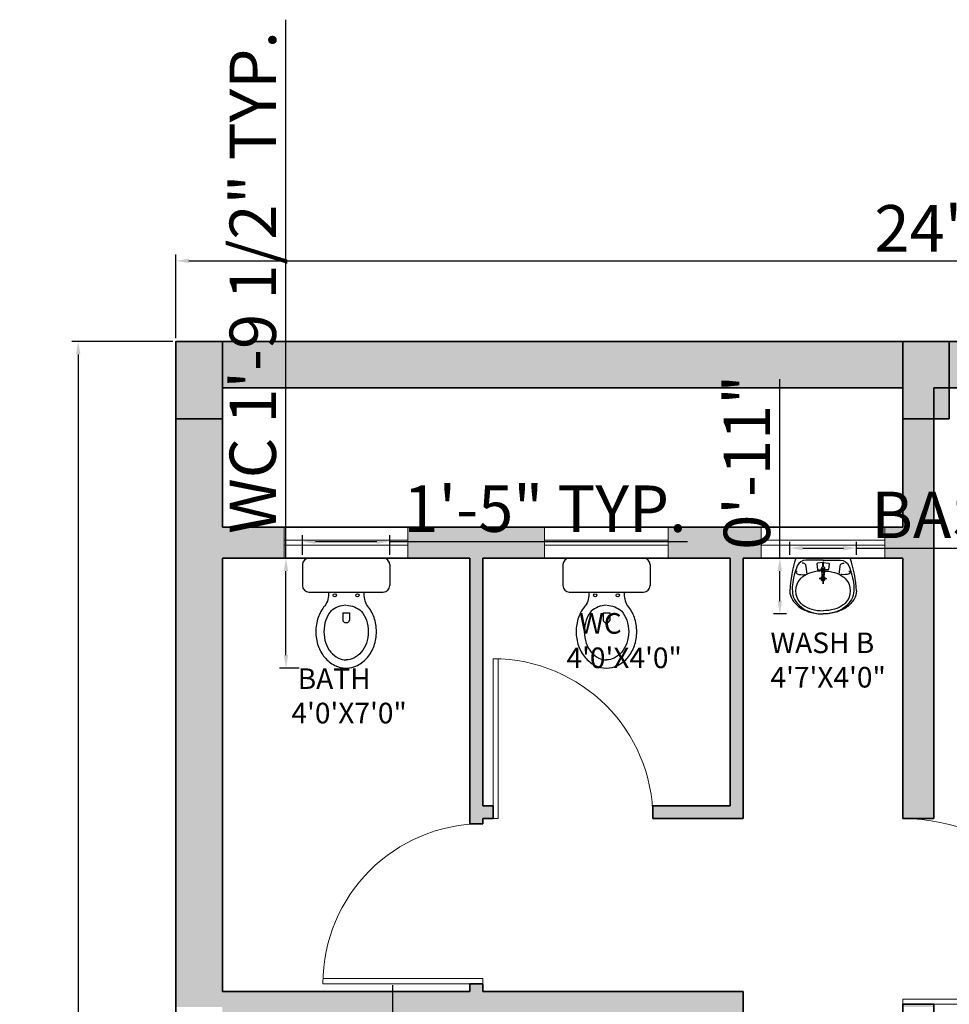
# Model space of a CAD drawing. Units: inches. Extents: x 3148 to 3962, y 1142 to 1671.
# Tile 3 of 9: x 3164 to 3344, y 1426 to 1617. Entities that reach past the tile are written whole.
import ezdxf

# ---------------------------------------------------------------- set-up
doc = ezdxf.new("R2010")
doc.units = ezdxf.units.IN
for name, color, linetype, lineweight in [('A-ANNO-DIMS', 2, 'Continuous', 18), ('A-AREA-IDEN', 7, 'Continuous', 18), ('A-COLS', 1, 'Continuous', 35), ('A-DOOR', 3, 'Continuous', 18), ('A-FLOR-FIXT', 21, 'Continuous', 18), ('A-GLAZ', 4, 'Continuous', 18), ('A-WALL', 7, 'Continuous', 35)]:
    doc.layers.add(name, color=color, linetype=linetype, lineweight=lineweight)
doc.layers.add('A-WALL-PATT', color=252, linetype='Continuous', lineweight=13, true_color=0x939598)
doc.layers.add('NOI-THAT-WC', color=11, linetype='Continuous')
doc.layers.add('THIET-BI', color=21, linetype='Continuous')
doc.styles.get("Standard").update_dxf_attribs({"font": 'arial.ttf'})
doc.dimstyles.new('ISO-25', dxfattribs={"dimtxt": 9, "dimasz": 2.5, "dimexe": 1.25, "dimexo": 0.625, "dimtad": 1, "dimdec": 1, "dimlunit": 3, "dimtxsty": 'Standard', "dimcen": 2.5, "dimadec": 0, "dimazin": 0, "dimtfac": 1, "dimtdec": 1, "dimtmove": 0, "dimatfit": 3, "dimfxl": 1, "dimarcsym": 0})

# ---------------------------------------------------------------- blocks, each defined once
blk = doc.blocks.new('A$C405E1C99')
at = {"layer": 'NOI-THAT-WC'}
for p, q in [((50, 460.7), (274.8, 460.7)), ((500, 460.7), (275.2, 460.7)), ((260.4, 373.8), (268.6, 307)), ((268.6, 307), (271.6, 376.3)), ((271.6, 376.3), (276.2, 376.3)), ((278.4, 376.3), (273.8, 376.3)), ((274.8, 249.7), (274.8, 327.3)), ((281.4, 307), (278.4, 376.3)), ((289.6, 373.8), (281.4, 307)), ((274.8, 291.6), (243.7, 291.6)), ((243.7, 291.6), (307.3, 291.6)), ((274.8, 251.3), (274.8, 324.2)), ((274.8, 291.6), (274.8, 251.3)), ((274.8, 291.6), (274.8, 249.7))]:
    blk.add_line(p, q, dxfattribs=at)
for points in [[(276.3, 443.6), (131.9, 443.6, 0.302606), (62.1, 397.1, 0.072962), (21.7, 238.9, 0.052091), (21.7, 190.5, 0.436057)], [(142.8, 325.8), (135, 395.6, 0.459808), (100.9, 418.8, 0.64626)], [(274.9, 425.6), (228.7, 419.7, 0.368294), (223.8, 414.3), (230.2, 367.7, 0.407548), (234.6, 364.2), (270, 364.2)], [(271.9, 388.9), (271.9, 425.2, -0.489286), (275.3, 427.9, -0.411473)], [(273.7, 443.6), (418.1, 443.6, -0.302606), (487.9, 397.1, -0.072962), (528.3, 238.9, -0.052091), (528.3, 190.5, -0.436057)], [(278.1, 388.9), (278.1, 425.2, 0.489286), (274.7, 427.9, 0.411473)], [(275.1, 425.6), (321.3, 419.7, -0.368294), (326.2, 414.3), (319.8, 367.7, -0.407548), (315.4, 364.2), (280, 364.2)], [(407.2, 325.8), (415, 395.6, -0.459808), (449.1, 418.8, -0.64626)], [(62.1, 355.2, 0.714157), (60.5, 332, 0.14855), (121.1, 325.8, -0.307941), (131.9, 321.1, 0.108948)], [(275, 355.2, 0.000185), (274.8, 355.2, 0.070372), (181.2, 342, 0.082088), (107.9, 307.1, 0.036954), (86.9, 290, 0.134876)], [(275, 355.2, -0.000185), (275.2, 355.2, -0.070372), (368.8, 342, -0.082088), (442.1, 307.1, -0.036954), (463.1, 290, -0.134876)], [(487.9, 355.2, -0.714157), (489.5, 332, -0.14855), (428.9, 325.8, 0.307941), (418.1, 321.1, -0.108948)], [(0, 190.8, 0.000665), (0, 190.4, 0.13527), (19.1, 121.4, 0.106902), (80.6, 55.6, 0.081908), (166, 15.2, 0.070137), (275, 0, 0.070137)], [(21.7, 190.8, 0.000567), (21.7, 190.5, 0.126238), (39.8, 120.4, 0.105991), (96, 55.7, 0.086052), (175.3, 15.1, 0.075833), (275, 0, 0.075833)], [(550, 190.8, -0.000665), (550, 190.4, -0.13527), (530.9, 121.4, -0.106902), (469.4, 55.6, -0.081908), (384, 15.2, -0.070137), (275, 0, -0.070137)], [(528.3, 190.8, -0.000567), (528.3, 190.5, -0.126238), (510.2, 120.4, -0.105991), (454, 55.7, -0.086052), (374.7, 15.1, -0.075833), (275, 0, -0.075833)], [(86.9, 91.6, 0.036954), (107.9, 74.5, 0.082088), (181.2, 39.6, 0.070372), (274.8, 26.4, 0.070372)], [(463.1, 91.6, -0.036954), (442.1, 74.5, -0.082088), (368.8, 39.6, -0.070372), (275.2, 26.4, -0.070372)], [(274.8, 26.4, 0.000185), (275, 26.4, 0.082088)], [(275.2, 26.4, -0.000185), (275, 26.4, -0.082088)], [(275, 0), (275, 0, 0.075833)], [(275, 0), (275, 0, 0.070137)]]:
    blk.add_lwpolyline(points, format="xyb", dxfattribs=at)
for centre, radius, start, end in [((1008.2, 143.6), 1009.3, 161.68953, 177.32082), ((-458.2, 143.6), 1009.3, 2.67918, 18.31047), ((274.9, 375), 14.5, 89.63157, 184.84688), ((275.1, 375), 14.5, 355.15312, 90.36843), ((189.4, 190.8), 142, 136.19016, 223.80984), ((274.8, 291.6), 17.3, 89.17695, 270.82305), ((274.8, 291.6), 12.8, 88.88475, 271.11525), ((275.2, 291.6), 17.3, 269.17695, 90.82305), ((275.2, 291.6), 12.8, 268.88475, 91.11525), ((360.6, 190.8), 142, 316.19016, 43.80984)]:
    blk.add_arc(centre, radius, start, end, dxfattribs=at)
blk = doc.blocks.new('A$C07D86673')
at = {"layer": 'THIET-BI'}
for p, q in [((40, 680), (500, 680)), ((0, 640), (0, 510)), ((540, 640), (540, 510)), ((40, 470), (500, 470)), ((158.6, 470), (158.6, 470)), ((250, 342.2), (290, 342.2)), ((250, 342.2), (250, 294.3)), ((290, 342.2), (290, 294.3)), ((251.5, 290.7), (259.5, 282.7)), ((259.5, 282.7), (280.5, 282.7)), ((280.5, 282.7), (288.5, 290.7))]:
    blk.add_line(p, q, dxfattribs=at)
for points in [[(158.6, 470, -0.215497), (137.4, 384.1, 0.09084), (97.2, 312.9, 0.083285), (82.5, 225, 0.083285), (97.2, 137.1, 0.09084), (137.4, 65.9, 0.104065), (200, 16.4, 0.115836), (270, 0, 0.115836), (340, 16.4, 0.104065), (402.6, 65.9, 0.09084), (442.8, 137.1, 0.083285), (457.5, 225, 0.083285)], [(457.5, 225, 0.083285), (442.8, 312.9, 0.09084), (402.6, 384.1, -0.156524), (381.4, 470)], [(268.2, 388.7, 0.171753), (175.8, 352.1, 0.09084), (144.5, 296.5, 0.083285), (132.5, 225, 0.083285), (144.5, 153.5, 0.09084), (175.8, 97.9, 0.104065), (222.3, 61.2, 0.115836), (270, 50, 0.115836)], [(271.8, 388.7, -0.171753), (364.2, 352.1, -0.09084), (395.5, 296.5, -0.083285), (407.5, 225, -0.083285), (395.5, 153.5, -0.09084), (364.2, 97.9, -0.104065), (317.7, 61.2, -0.115836), (270, 50, -0.115836)]]:
    blk.add_lwpolyline(points, format="xyb", dxfattribs=at)
for centre in [(200, 450), (340, 450)]:
    blk.add_circle(centre, 10, dxfattribs=at)
for centre, radius, start, end in [((40, 640), 40, 90, 180), ((500, 640), 40, 0, 90), ((40, 510), 40, 180, 270), ((500, 510), 40, 270, 0), ((255, 294.3), 5, 180, 225), ((285, 294.3), 5, 315, 0)]:
    blk.add_arc(centre, radius, start, end, dxfattribs=at)
blk = doc.blocks.new('*D42')
at = {"layer": 'A-ANNO-DIMS', "color": 0, "lineweight": -2, "transparency": 16777216}
for p, q in [((3194.04, 1555.42), (3194.04, 1571.69)), ((3482.04, 1555.42), (3482.04, 1571.69)), ((3196.54, 1570.44), (3479.54, 1570.44))]:
    blk.add_line(p, q, dxfattribs=at)
at = {"layer": 'A-ANNO-DIMS', "color": 0, "transparency": 16777216}
for points in [[(3196.54, 1570.86), (3196.54, 1570.02), (3194.04, 1570.44)], [(3479.54, 1570.86), (3479.54, 1570.02), (3482.04, 1570.44)]]:
    blk.add_solid(points, dxfattribs=at)
at = {"layer": 'Defpoints', "color": 0, "transparency": 16777216}
for p in [(3482.04, 1570.44), (3194.04, 1554.8), (3482.04, 1554.8)]:
    blk.add_point(p, dxfattribs=at)
at = {"layer": 'A-ANNO-DIMS', "color": 0, "transparency": 16777216, "insert": (3338.04, 1575.58), "char_height": 9, "attachment_point": 5}
blk.add_mtext("24'", dxfattribs=at)
blk = doc.blocks.new('*D43')
at = {"layer": 'A-ANNO-DIMS', "color": 0, "lineweight": -2, "transparency": 16777216}
for p, q in [((3193.42, 1554.8), (3173.83, 1554.8)), ((3175.08, 1552.3), (3175.08, 1200.3)), ((3193.42, 1197.8), (3173.83, 1197.8))]:
    blk.add_line(p, q, dxfattribs=at)
at = {"layer": 'A-ANNO-DIMS', "color": 0, "transparency": 16777216}
for points in [[(3174.66, 1552.3), (3175.5, 1552.3), (3175.08, 1554.8)], [(3174.66, 1200.3), (3175.5, 1200.3), (3175.08, 1197.8)]]:
    blk.add_solid(points, dxfattribs=at)
at = {"layer": 'Defpoints', "color": 0, "transparency": 16777216}
for p in [(3194.04, 1554.8), (3175.08, 1197.8), (3194.04, 1197.8)]:
    blk.add_point(p, dxfattribs=at)
at = {"layer": 'A-ANNO-DIMS', "color": 0, "transparency": 16777216, "insert": (3169.86, 1376.3), "char_height": 9, "attachment_point": 5, "rotation": 90}
blk.add_mtext('29\'-9"', dxfattribs=at)
blk = doc.blocks.new('DOOR-SWING-31')
for p, q in [((0, 31), (0, 0)), ((1, 31), (1, 0)), ((0, 0), (1, 0))]:
    blk.add_line(p, q)
blk.add_arc((0, 0), 31, 0, 90)
blk = doc.blocks.new('DOOR-SWING-36')
for p, q in [((35.99, 1), (0, 1)), ((0, 0), (0, 1)), ((36, 0), (0, 0))]:
    blk.add_line(p, q)
blk.add_arc((0, 0), 36, 0, 90)
blk = doc.blocks.new('WIN-24')
for p, q in [((0, 6), (0, 0)), ((24, 6), (24, 0)), ((24, 3.5), (0, 3.5)), ((24, 2.5), (0, 2.5))]:
    blk.add_line(p, q)
blk = doc.blocks.new('COL-9X15')
h = blk.add_hatch(color=256)
h.dxf.hatch_style = 1
h.paths.add_polyline_path([(9, 15), (0, 15), (0, 0), (9, 0)])
blk.add_lwpolyline([(9, 0), (9, 15), (0, 15), (0, 0)], close=True)
blk = doc.blocks.new('*D90')
at = {"layer": 'A-ANNO-DIMS', "color": 0, "lineweight": -2, "transparency": 16777216}
for p, q in [((3215.38, 1512.8), (3215.38, 1617.19)), ((3217.96, 1512.8), (3214.13, 1512.8)), ((3215.38, 1493.99), (3215.38, 1510.3)), ((3217.96, 1491.49), (3214.13, 1491.49))]:
    blk.add_line(p, q, dxfattribs=at)
at = {"layer": 'A-ANNO-DIMS', "color": 0, "transparency": 16777216}
for points in [[(3214.97, 1510.3), (3215.8, 1510.3), (3215.38, 1512.8)], [(3214.97, 1493.99), (3215.8, 1493.99), (3215.38, 1491.49)]]:
    blk.add_solid(points, dxfattribs=at)
at = {"layer": 'Defpoints', "color": 0, "transparency": 16777216}
for p in [(3215.38, 1512.8), (3218.58, 1512.8), (3218.58, 1491.49)]:
    blk.add_point(p, dxfattribs=at)
at = {"layer": 'A-ANNO-DIMS', "color": 0, "transparency": 16777216, "insert": (3210.11, 1566.24), "char_height": 9, "attachment_point": 5, "rotation": 90}
blk.add_mtext('WC 1\'-9 1/2" TYP.', dxfattribs=at)
blk = doc.blocks.new('*D91')
at = {"layer": 'A-ANNO-DIMS', "color": 0, "lineweight": -2, "transparency": 16777216}
for p, q in [((3218.58, 1513.42), (3218.58, 1517.25)), ((3221.08, 1516), (3233, 1516)), ((3235.5, 1513.42), (3235.5, 1517.25)), ((3235.5, 1516), (3293.27, 1516))]:
    blk.add_line(p, q, dxfattribs=at)
at = {"layer": 'A-ANNO-DIMS', "color": 0, "transparency": 16777216}
for points in [[(3221.08, 1516.41), (3221.08, 1515.58), (3218.58, 1516)], [(3233, 1516.41), (3233, 1515.58), (3235.5, 1516)]]:
    blk.add_solid(points, dxfattribs=at)
at = {"layer": 'Defpoints', "color": 0, "transparency": 16777216}
for p in [(3235.5, 1516), (3218.58, 1512.8), (3235.5, 1512.8)]:
    blk.add_point(p, dxfattribs=at)
at = {"layer": 'A-ANNO-DIMS', "color": 0, "transparency": 16777216, "insert": (3265.63, 1521.22), "char_height": 9, "attachment_point": 5}
blk.add_mtext('1\'-5" TYP.', dxfattribs=at)
blk = doc.blocks.new('*D102')
at = {"layer": 'A-ANNO-DIMS', "color": 0, "lineweight": -2, "transparency": 16777216}
for p, q in [((3236.08, 1276.67), (3236.08, 1430.01)), ((3238.82, 1276.67), (3234.83, 1276.67)), ((3236.08, 1256.73), (3236.08, 1274.17)), ((3238.82, 1254.23), (3234.83, 1254.23))]:
    blk.add_line(p, q, dxfattribs=at)
at = {"layer": 'A-ANNO-DIMS', "color": 0, "transparency": 16777216}
for points in [[(3235.66, 1274.17), (3236.49, 1274.17), (3236.08, 1276.67)], [(3235.66, 1256.73), (3236.49, 1256.73), (3236.08, 1254.23)]]:
    blk.add_solid(points, dxfattribs=at)
at = {"layer": 'Defpoints', "color": 0, "transparency": 16777216}
for p in [(3236.08, 1276.67), (3239.44, 1276.67), (3239.44, 1254.23)]:
    blk.add_point(p, dxfattribs=at)
at = {"layer": 'A-ANNO-DIMS', "color": 0, "transparency": 16777216, "insert": (3230.8, 1354.59), "char_height": 9, "attachment_point": 5, "rotation": 90}
blk.add_mtext('COFFEE TABLE 1\'-10 1/2"', dxfattribs=at)
blk = doc.blocks.new('*D110')
at = {"layer": 'A-ANNO-DIMS', "color": 0, "lineweight": -2, "transparency": 16777216}
for p, q in [((3313.1, 1513.42), (3313.1, 1515.99)), ((3326.01, 1513.42), (3326.01, 1515.99)), ((3315.6, 1514.74), (3323.51, 1514.74)), ((3326.01, 1514.74), (3394.51, 1514.74))]:
    blk.add_line(p, q, dxfattribs=at)
at = {"layer": 'A-ANNO-DIMS', "color": 0, "transparency": 16777216}
for points in [[(3315.6, 1515.15), (3315.6, 1514.32), (3313.1, 1514.74)], [(3323.51, 1515.15), (3323.51, 1514.32), (3326.01, 1514.74)]]:
    blk.add_solid(points, dxfattribs=at)
at = {"layer": 'Defpoints', "color": 0, "transparency": 16777216}
for p in [(3326.01, 1514.74), (3313.1, 1512.8), (3326.01, 1512.8)]:
    blk.add_point(p, dxfattribs=at)
at = {"layer": 'A-ANNO-DIMS', "color": 0, "transparency": 16777216, "insert": (3361.51, 1520.01), "char_height": 9, "attachment_point": 5}
blk.add_mtext('BASIN 1\'-1"', dxfattribs=at)
blk = doc.blocks.new('*D111')
at = {"layer": 'A-ANNO-DIMS', "color": 0, "lineweight": -2, "transparency": 16777216}
for p, q in [((3311.17, 1512.8), (3311.17, 1547.47)), ((3312.48, 1512.8), (3309.92, 1512.8)), ((3311.17, 1504.48), (3311.17, 1510.3)), ((3312.48, 1501.98), (3309.92, 1501.98))]:
    blk.add_line(p, q, dxfattribs=at)
at = {"layer": 'A-ANNO-DIMS', "color": 0, "transparency": 16777216}
for points in [[(3310.75, 1510.3), (3311.58, 1510.3), (3311.17, 1512.8)], [(3310.75, 1504.48), (3311.58, 1504.48), (3311.17, 1501.98)]]:
    blk.add_solid(points, dxfattribs=at)
at = {"layer": 'Defpoints', "color": 0, "transparency": 16777216}
for p in [(3311.17, 1512.8), (3313.1, 1512.8), (3313.1, 1501.98)]:
    blk.add_point(p, dxfattribs=at)
at = {"layer": 'A-ANNO-DIMS', "color": 0, "transparency": 16777216, "insert": (3305.94, 1531.38), "char_height": 9, "attachment_point": 5, "rotation": 90}
blk.add_mtext('0\'-11"', dxfattribs=at)

msp = doc.modelspace()

# ---------------------------------------------------------------- hatches: boundary and pattern name
at = {"layer": 'A-WALL-PATT'}
h = msp.add_hatch(color=256, dxfattribs=at)
h.dxf.hatch_style = 1
h.paths.add_polyline_path([(3203.04, 1410.8), (3194.04, 1410.8), (3194.04, 1296.8), (3203.04, 1296.8), (3203.04, 1300.86)])
h.paths.add_polyline_path([(3203.04, 1281.8), (3194.04, 1281.8), (3194.04, 1212.8), (3203.04, 1212.8)])
h.paths.add_polyline_path([(3326.04, 1206.8), (3203.04, 1206.8), (3203.04, 1197.8), (3326.04, 1197.8)])
h.paths.add_polyline_path([(3341.04, 1362.8), (3335.04, 1362.8), (3335.04, 1290.8), (3341.04, 1290.8)])
h.paths.add_polyline_path([(3341.04, 1207.8), (3335.04, 1207.8), (3335.04, 1206.8), (3341.04, 1206.8)])
h.paths.add_polyline_path([(3341.04, 1259.8), (3335.04, 1259.8), (3335.04, 1255.8), (3341.04, 1255.8)])
h.paths.add_polyline_path([(3341.04, 1281.8), (3335.04, 1281.8), (3335.04, 1277.8), (3341.04, 1277.8)])
h.paths.add_polyline_path([(3377.04, 1287.8), (3350.04, 1287.8), (3350.04, 1281.8), (3377.04, 1281.8)])
h.paths.add_polyline_path([(3473.04, 1287.8), (3445.04, 1287.8), (3437.04, 1287.8), (3437.04, 1281.8), (3473.04, 1281.8)])
h.paths.add_polyline_path([(3482.04, 1313.3), (3473.04, 1313.3), (3473.04, 1296.8), (3482.04, 1296.8)])
h.paths.add_polyline_path([(3482.04, 1410.8), (3473.04, 1410.8), (3473.04, 1385.3), (3482.04, 1385.3)])
h.paths.add_polyline_path([(3473.04, 1416.8), (3344.04, 1416.8), (3344.04, 1410.8), (3473.04, 1410.8)])
h.paths.add_polyline_path([(3482.04, 1445.3), (3473.04, 1445.3), (3473.04, 1425.8), (3482.04, 1425.8)])
h.paths.add_polyline_path([(3341.04, 1426.3), (3335.04, 1426.3), (3335.04, 1425.8), (3341.04, 1425.8)])
h.paths.add_polyline_path([(3304.04, 1428.8), (3253.54, 1428.8), (3253.54, 1430.3), (3251.04, 1430.3), (3251.04, 1428.8), (3203.04, 1428.8), (3203.04, 1512.8), (3215.04, 1512.8), (3215.04, 1518.8), (3203.04, 1518.8), (3203.04, 1539.8), (3194.04, 1539.8), (3194.04, 1425.8), (3203.04, 1425.8), (3203.04, 1422.8), (3304.04, 1422.8)])
h.paths.add_polyline_path([(3265.54, 1518.8), (3239.04, 1518.8), (3239.04, 1512.8), (3251.04, 1512.8), (3251.04, 1461.3), (3253.54, 1461.3), (3253.54, 1462.3), (3255.54, 1462.3), (3255.54, 1464.8), (3253.54, 1464.8), (3253.54, 1512.8), (3265.54, 1512.8)], flags=17)
h.paths.add_polyline_path([(3307.54, 1518.8), (3289.54, 1518.8), (3289.54, 1512.8), (3301.54, 1512.8), (3301.54, 1464.8), (3286.54, 1464.8), (3286.54, 1462.3), (3304.04, 1462.3), (3304.04, 1512.8), (3307.54, 1512.8)])
h.paths.add_polyline_path([(3341.04, 1539.8), (3335.04, 1539.8), (3335.04, 1518.8), (3331.54, 1518.8), (3331.54, 1512.8), (3335.04, 1512.8), (3335.04, 1462.3), (3341.04, 1462.3)])
h.paths.add_polyline_path([(3335.04, 1554.8), (3203.04, 1554.8), (3203.04, 1545.8), (3335.04, 1545.8)])
h.paths.add_polyline_path([(3473.04, 1554.8), (3344.04, 1554.8), (3344.04, 1545.8), (3362.94, 1545.8), (3473.04, 1545.8)])
h.paths.add_polyline_path([(3482.04, 1539.8), (3473.04, 1539.8), (3473.04, 1517.3), (3482.04, 1517.3)])

# ---------------------------------------------------------------- linework, layer by layer
at = {"layer": 'A-WALL'}
for p, q in [((3194.04, 1197.8), (3194.04, 1554.8)), ((3194.04, 1554.8), (3482.04, 1554.8)), ((3203.04, 1545.8), (3335.04, 1545.8)), ((3203.04, 1518.8), (3203.04, 1545.8)), ((3335.04, 1545.8), (3335.04, 1518.8)), ((3341.04, 1545.8), (3341.04, 1462.3)), ((3341.04, 1545.8), (3473.04, 1545.8)), ((3335.04, 1518.8), (3203.04, 1518.8)), ((3203.04, 1428.8), (3203.04, 1512.8)), ((3251.04, 1512.8), (3203.04, 1512.8)), ((3251.04, 1461.3), (3251.04, 1512.8)), ((3301.54, 1512.8), (3253.54, 1512.8)), ((3253.54, 1464.8), (3253.54, 1512.8)), ((3301.54, 1464.8), (3301.54, 1512.8)), ((3335.04, 1512.8), (3304.04, 1512.8)), ((3304.04, 1462.3), (3304.04, 1512.8)), ((3335.04, 1512.8), (3335.04, 1462.3)), ((3255.54, 1464.8), (3253.54, 1464.8)), ((3255.54, 1462.3), (3255.54, 1464.8)), ((3301.54, 1464.8), (3286.54, 1464.8)), ((3286.54, 1462.3), (3286.54, 1464.8)), ((3253.54, 1461.3), (3253.54, 1462.3)), ((3255.54, 1462.3), (3253.54, 1462.3)), ((3304.04, 1462.3), (3286.54, 1462.3)), ((3335.04, 1462.3), (3341.04, 1462.3)), ((3253.54, 1461.3), (3251.04, 1461.3)), ((3251.04, 1428.8), (3251.04, 1430.3)), ((3253.54, 1430.3), (3251.04, 1430.3)), ((3253.54, 1428.8), (3253.54, 1430.3)), ((3251.04, 1428.8), (3203.04, 1428.8)), ((3304.04, 1428.8), (3253.54, 1428.8)), ((3304.04, 1422.8), (3304.04, 1428.8)), ((3335.04, 1426.3), (3341.04, 1426.3)), ((3335.04, 1426.3), (3335.04, 1410.8)), ((3341.04, 1426.3), (3341.04, 1416.8))]:
    msp.add_line(p, q, dxfattribs=at)

# ---------------------------------------------------------------- block references
at = {"layer": 'A-COLS'}
for p in [(3194.04, 1539.8), (3335.04, 1539.8)]:
    msp.add_blockref('COL-9X15', p, dxfattribs=at)
at = {"layer": 'A-DOOR'}
for name, p in [('DOOR-SWING-31', (3255.54, 1462.3)), ('DOOR-SWING-36', (3335.04, 1426.3))]:
    msp.add_blockref(name, p, dxfattribs=at)
at = {"layer": 'A-DOOR', "rotation": 89.99999999999801}
msp.add_blockref('DOOR-SWING-31', (3253.54, 1430.3), dxfattribs=at)
at = {"layer": 'A-FLOR-FIXT'}
for name, p, xscale, yscale, zscale in [('A$C07D86673', (3218.58, 1491.49), 0.0313378757302851, 0.0313378757302851, 0.0313378757302851), ('A$C07D86673', (3269.08, 1491.49), 0.0313378757302851, 0.0313378757302851, 0.0313378757302851), ('A$C405E1C99', (3313.1, 1501.98), 0.0234753834705155, 0.0234753834705155, 0.0234753834705155)]:
    msp.add_blockref(name, p, dxfattribs=dict(at, xscale=xscale, yscale=yscale, zscale=zscale))
at = {"layer": 'A-GLAZ', "rotation": 180}
msp.add_blockref('WIN-24', (3239.04, 1518.8), dxfattribs=at)
at = {"layer": 'A-GLAZ'}
for p in [(3265.54, 1512.8), (3307.54, 1512.8)]:
    msp.add_blockref('WIN-24', p, dxfattribs=at)

# ---------------------------------------------------------------- texts
at = {"layer": 'A-AREA-IDEN', "char_height": 4, "attachment_point": 1}
for s, insert in [('  WC\\P4\'0\'X4\'0"', (3269.78, 1502.14)), ('WASH B\\P4\'7\'X4\'0"', (3309.35, 1498.38)), (' BATH\\P4\'0\'X7\'0"', (3216.43, 1491.43))]:
    msp.add_mtext_dynamic_manual_height_columns(s, width=77.9518, gutter_width=12.5, heights=[0], dxfattribs=dict(at, insert=insert))

# ---------------------------------------------------------------- dimensions: what is measured, and where the dimension line sits
at = {"layer": 'A-ANNO-DIMS'}
for base, p1, p2, text, picture, middle in [((3215.38, 1512.8), (3218.58, 1491.49), (3218.58, 1512.8), 'WC <> TYP.', '*D90', (3210.11, 1566.24)), ((3236.08, 1276.67), (3239.44, 1254.23), (3239.44, 1276.67), 'COFFEE TABLE <>', '*D102', (3230.8, 1354.59))]:
    dim = msp.add_linear_dim(base=base, p1=p1, p2=p2, angle=90, text=text, dimstyle='ISO-25', override={"dimdec": 1, "dimlfac": 1, "dimrnd": 0, "dimzin": 1, "dimdsep": 46, "dimlunit": 4, "dimfrac": 2}, dxfattribs=at)
    dim.commit()
    dim.dimension.update_dxf_attribs({"geometry": picture, "text_midpoint": middle})
dim = msp.add_linear_dim(base=(3482.04, 1570.44), p1=(3194.04, 1554.8), p2=(3482.04, 1554.8), dimstyle='ISO-25', override={"dimclrd": 0, "dimclre": 0, "dimclrt": 0}, dxfattribs=at)
dim.commit()
dim.dimension.update_dxf_attribs({"geometry": '*D42', "text_midpoint": (3338.04, 1575.58)})
for base, p1, p2, override, picture, middle in [((3175.08, 1197.8), (3194.04, 1554.8), (3194.04, 1197.8), {"dimclrd": 0, "dimclre": 0, "dimclrt": 0}, '*D43', (3169.86, 1376.3)), ((3311.17, 1512.8), (3313.1, 1501.98), (3313.1, 1512.8), {"dimdec": 1, "dimlfac": 1, "dimrnd": 0, "dimzin": 1, "dimdsep": 46, "dimlunit": 4, "dimfrac": 2}, '*D111', (3305.94, 1531.38))]:
    dim = msp.add_linear_dim(base=base, p1=p1, p2=p2, angle=90, dimstyle='ISO-25', override=override, dxfattribs=at)
    dim.commit()
    dim.dimension.update_dxf_attribs({"geometry": picture, "text_midpoint": middle})
for base, p1, p2, text, picture, middle in [((3235.5, 1516), (3218.58, 1512.8), (3235.5, 1512.8), '<> TYP.', '*D91', (3265.63, 1521.22)), ((3326.01, 1514.74), (3313.1, 1512.8), (3326.01, 1512.8), 'BASIN <>', '*D110', (3361.51, 1520.01))]:
    dim = msp.add_linear_dim(base=base, p1=p1, p2=p2, text=text, dimstyle='ISO-25', override={"dimdec": 1, "dimlfac": 1, "dimrnd": 0, "dimzin": 1, "dimdsep": 46, "dimlunit": 4, "dimfrac": 2}, dxfattribs=at)
    dim.commit()
    dim.dimension.update_dxf_attribs({"geometry": picture, "text_midpoint": middle})

doc.saveas('drawing.dxf')
